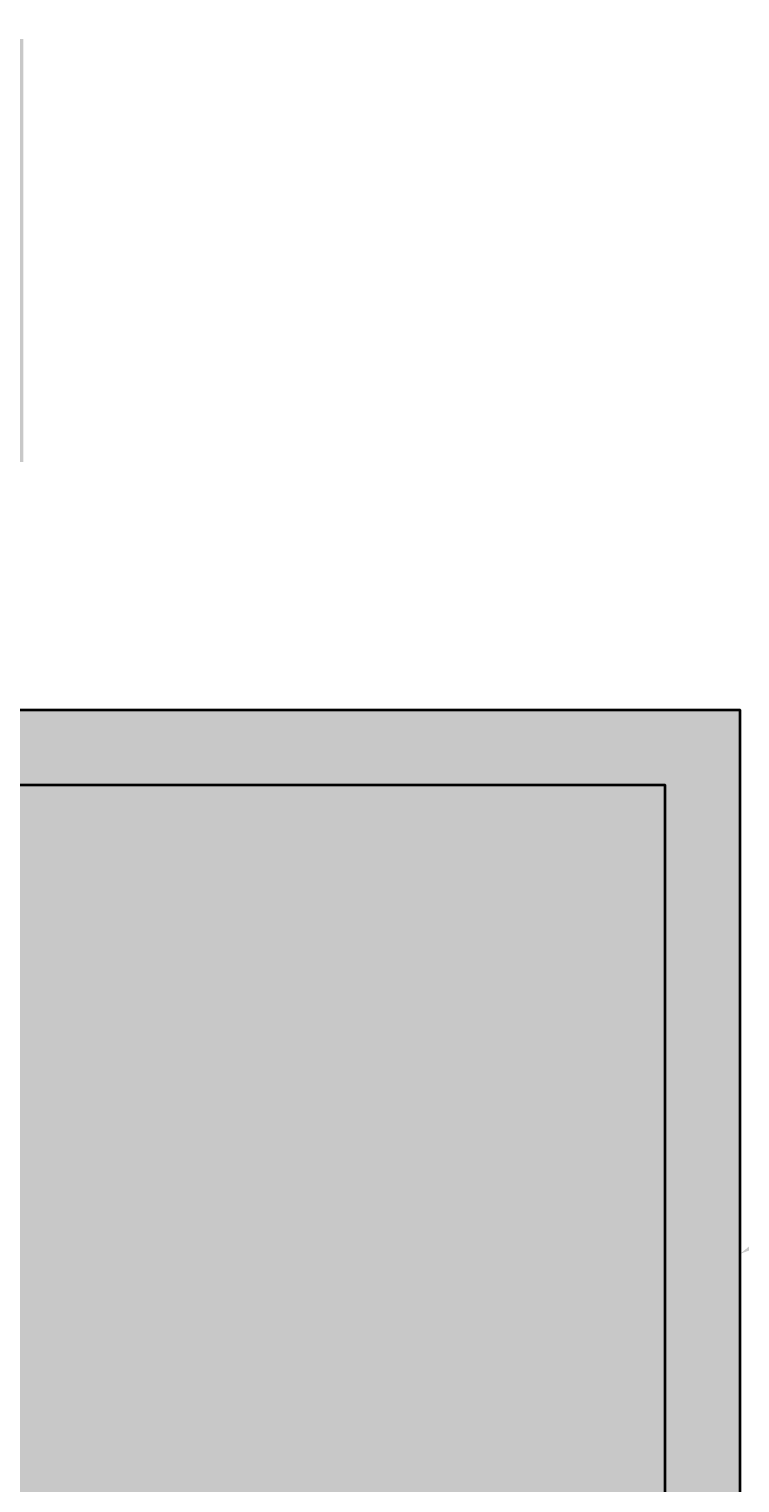
# Model space of a CAD drawing. Units: millimetres. Extents: x -11 to 280, y -4 to 208.
# Tile 16 of 55: x 52 to 66, y 164 to 193. Entities that reach past the tile are written whole.
import ezdxf
from ezdxf import colors
from ezdxf.entities.mleader import LeaderData, LeaderLine
from ezdxf.math import Vec2, Vec3

# ---------------------------------------------------------------- set-up
doc = ezdxf.new("R2010")
doc.units = ezdxf.units.MM
for name, color, linetype, lineweight in [('M-ANNO-TEXT', 7, 'Continuous', 18), ('M-DIMS', 2, 'Continuous', 18), ('M-HYDR-EQPM', 7, 'Continuous', 35), ('M-HYDR-EQPM-PATT', 252, 'Continuous', 13)]:
    doc.layers.add(name, color=color, linetype=linetype, lineweight=lineweight)
doc.styles.get("Standard").update_dxf_attribs({"font": 'arial.ttf'})
doc.dimstyles.get("Standard").update_dxf_attribs({"dimtxt": 0.18, "dimasz": 0.18, "dimexe": 0.18, "dimexo": 0.0625, "dimgap": 0.09, "dimtad": 0, "dimtih": 1, "dimtoh": 1, "dimdec": 4, "dimzin": 0, "dimdsep": 46, "dimtxsty": 'Standard', "dimcen": 0.09, "dimadec": 0, "dimazin": 0, "dimtfac": 1, "dimtdec": 4, "dimtofl": 0, "dimtmove": 0, "dimatfit": 3, "dimfxl": 1, "dimtolj": 1, "dimtzin": 0, "dimarcsym": 0})

# ---------------------------------------------------------------- blocks, each defined once
blk = doc.blocks.new('*D5')
at = {"layer": 'Defpoints', "color": 0, "transparency": 16777216}
for p in [(24.759, 192.645), (-10.087, 11.435), (261.686, 11.435)]:
    blk.add_point(p, dxfattribs=at)
at = {"layer": 'M-DIMS', "color": 0, "lineweight": -2, "transparency": 16777216}
for p, q in [((24.696, 192.645), (-10.267, 192.645)), ((-10.087, 192.465), (-10.087, 102.222)), ((-10.087, 11.615), (-10.087, 101.858)), ((261.624, 11.435), (-10.267, 11.435))]:
    blk.add_line(p, q, dxfattribs=at)
at = {"layer": 'M-DIMS', "color": 0, "transparency": 16777216}
for points in [[(-10.117, 192.465), (-10.057, 192.465), (-10.087, 192.645)], [(-10.117, 11.615), (-10.057, 11.615), (-10.087, 11.435)]]:
    blk.add_solid(points, dxfattribs=at)
at = {"layer": 'M-DIMS', "color": 0, "transparency": 16777216, "insert": (-10.087, 102.04), "char_height": 0.18, "attachment_point": 5}
blk.add_mtext('\\A1;181.2', dxfattribs=at)
blk = doc.blocks.new('*D9')
at = {"layer": 'Defpoints', "color": 0, "transparency": 16777216}
for p in [(78.827, 207.495), (31.006, 98.021), (78.827, 98.149)]:
    blk.add_point(p, dxfattribs=at)
at = {"layer": 'M-DIMS', "color": 0, "lineweight": -2, "transparency": 16777216}
for p, q in [((31.006, 98.084), (31.006, 207.675)), ((31.186, 207.495), (54.52, 207.495)), ((78.647, 207.495), (55.313, 207.495)), ((78.827, 98.212), (78.827, 207.675))]:
    blk.add_line(p, q, dxfattribs=at)
at = {"layer": 'M-DIMS', "color": 0, "transparency": 16777216}
for points in [[(31.186, 207.525), (31.186, 207.465), (31.006, 207.495)], [(78.647, 207.525), (78.647, 207.465), (78.827, 207.495)]]:
    blk.add_solid(points, dxfattribs=at)
at = {"layer": 'M-DIMS', "color": 0, "transparency": 16777216, "insert": (54.917, 207.495), "char_height": 0.18, "attachment_point": 5}
blk.add_mtext('\\A1;47.82', dxfattribs=at)

msp = doc.modelspace()

# ---------------------------------------------------------------- hatches: boundary and pattern name
at = {"layer": 'M-HYDR-EQPM-PATT'}
h = msp.add_hatch(color=256, dxfattribs=at)
h.set_gradient(color1=(153, 153, 0), color2=(255, 255, 0), tint=1, name='INVCYLINDER')
h.paths.add_polyline_path([(64.8875, 177.7412), (30.7015, 177.7412), (30.7015, 155.4768), (64.8875, 155.4768)])
h.paths.add_polyline_path([(52.0736, 184.1929), (52.0736, 192.645), (24.7588, 192.645), (24.7588, 184.1929), (34.0713, 184.1929), (34.0713, 179.2412), (35.5061, 179.2412), (35.5061, 185.6276), (26.1935, 185.6276), (26.1935, 191.2103), (50.6389, 191.2103), (50.6389, 185.6276), (41.792, 185.6276), (41.792, 179.2412), (43.2268, 179.2412), (43.2268, 184.1929)])
h = msp.add_hatch(color=256, dxfattribs=at)
h.set_gradient(color1=(153, 153, 0), color2=(153, 153, 0), tint=1, name='INVCYLINDER')
h.paths.add_polyline_path([(26.1935, 191.2103), (26.1935, 185.6276), (35.5061, 185.6276), (35.5061, 179.2412), (41.792, 179.2412), (41.792, 185.6276), (50.6389, 185.6276), (50.6389, 191.2103)])
h.paths.add_polyline_path([(29.2015, 153.9768), (66.3875, 153.9768), (66.3875, 179.2412), (29.2015, 179.2412)])
h.paths.add_polyline_path([(30.7015, 177.7412), (64.8875, 177.7412), (64.8875, 155.4768), (30.7015, 155.4768)], flags=16)

# ---------------------------------------------------------------- linework, layer by layer
at = {"layer": 'M-HYDR-EQPM'}
for points in [[(29.2015, 179.2412), (66.3875, 179.2412), (66.3875, 153.9768), (29.2015, 153.9768)], [(30.7015, 177.7412), (64.8875, 177.7412), (64.8875, 155.4768), (30.7015, 155.4768)]]:
    msp.add_lwpolyline(points, close=True, dxfattribs=at)

# ---------------------------------------------------------------- dimensions: what is measured, and where the dimension line sits
at = {"layer": 'M-DIMS'}
dim = msp.add_linear_dim(base=(78.8273, 207.495), p1=(31.0059, 98.0213), p2=(78.8273, 98.1491), dimstyle='Standard', override={"dimdec": 2, "dimlfac": 1, "dimrnd": 0, "dimzin": 0, "dimdsep": 46, "dimlunit": 2}, dxfattribs=at)
dim.commit()
dim.dimension.update_dxf_attribs({"geometry": '*D9', "text_midpoint": (54.9166, 207.495)})
dim = msp.add_linear_dim(base=(-10.0865, 11.4346), p1=(24.7588, 192.645), p2=(261.6863, 11.4346), angle=90, dimstyle='Standard', override={"dimdec": 1, "dimlfac": 1, "dimrnd": 0, "dimzin": 0, "dimdsep": 46, "dimlunit": 2}, dxfattribs=at)
dim.commit()
dim.dimension.update_dxf_attribs({"geometry": '*D5', "text_midpoint": (-10.0865, 102.0398)})

# ---------------------------------------------------------------- leaders
at = {"layer": 'M-ANNO-TEXT'}
ml = msp.add_multileader_mtext('Standard', dxfattribs=at)
ml.set_content('RESERVOIR', color=256)
ml.set_leader_properties()
ml.build(insert=Vec2(0, 0))
ctx = ml.context
ctx.base_point, ctx.plane_origin = Vec3(86.1452, 175.1554), Vec3(66.3875, 168.3671)
notes = []
notes.append((ctx, [(0, (1, 1, 0), (78.1452, 175.1554), (1, 0), 8, [(0, [(66.3875, 168.3671)], 0, [])])]))
ctx.mtext.insert, ctx.mtext.flow_direction = Vec3(88.1452, 177.1895), 5
for ctx, leaders in notes:
    for number, flags, end, landing, length, lines in leaders:
        leader = LeaderData()
        leader.index, (leader.has_last_leader_line, leader.has_dogleg_vector, leader.attachment_direction) = number, flags
        leader.last_leader_point, leader.dogleg_vector, leader.dogleg_length = Vec3(end), Vec3(landing), length
        for number, points, colour, breaks in lines:
            line = LeaderLine()
            line.index, line.vertices, line.color, line.breaks = number, Vec3.list(points), colors.encode_raw_color(colour), breaks
            leader.lines.append(line)
        ctx.leaders.append(leader)

doc.saveas('drawing.dxf')
